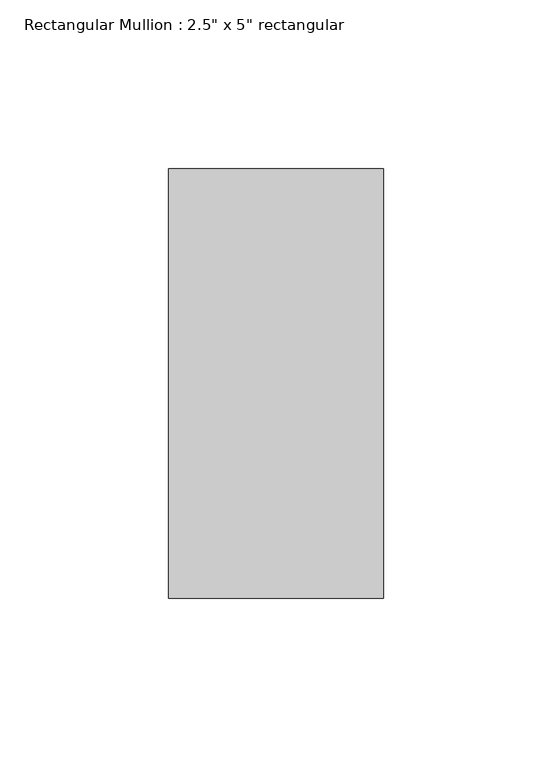
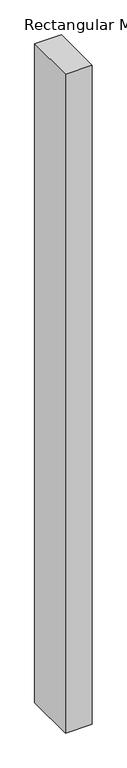
"""IFC4 building model written with IfcOpenShell, lengths in millimetres: member geometry."""

from ifc_helpers import new_model, si_unit, frame, origin, place, context, project, spatial, polyline, outline, extrude, source, transform, mapped, element, save


def member_ccb4fae7(model_context):
    return source(origin(), model_context, "Body", "SweptSolid", [
        extrude(outline(polyline([(31.75, 63.5), (31.75, -63.5), (-31.75, -63.5), (-31.75, 63.5), (31.75, 63.5)])), frame((0.0, 0.0, -1660.012385), z_axis=(0.0, 0.0, 1.0), x_axis=(1.0, 0.0, 0.0)), (0.0, 0.0, 1.0), 1660.012385),
    ])


if __name__ == "__main__":
    model = new_model("IFC4")
    model_context = context("Model", 3, world=origin())
    ifc_project = project(units=[si_unit("LENGTHUNIT", "METRE", prefix="MILLI")], contexts=[model_context])
    site = spatial("IfcSite", under=ifc_project)
    building = spatial("IfcBuilding", under=site)
    placement = place(None, origin())
    member_shape = member_ccb4fae7(model_context)
    element("IfcMember", 1, ObjectType="Rectangular Mullion : 2.5\" x 5\" rectangular", at=placement, inside=building, context=model_context, shape_type="MappedRepresentation", body=[
        mapped(member_shape, transform((0.0, 0.0, 0.0), x_axis=(1.0, 0.0, 0.0), y_axis=(0.0, 1.0, 0.0), z_axis=(0.0, 0.0, 1.0))),
    ])
    save(model, "model.ifc")

# Revit data of these elements
# Type "Rectangular Mullion : 2.5\" x 5\" rectangular"
#   built-in parameter 1007304 = 0.416667 (stored number, unit not read)
#   built-in parameter 1007301 = 0.104167 (stored number, unit not read)
#   built-in parameter 1007300 = 0.104167 (stored number, unit not read)
# Element 1 (IfcMember, "Rectangular Mullion : 2.5\" x 5\" rectangular")
#   Materials on its faces: "Aluminum"
# Materials
#   "Aluminum": class "Metal", colour RGB 247 247 247, transparency 0, Description = "Aluminum 6061", Cost = 0
